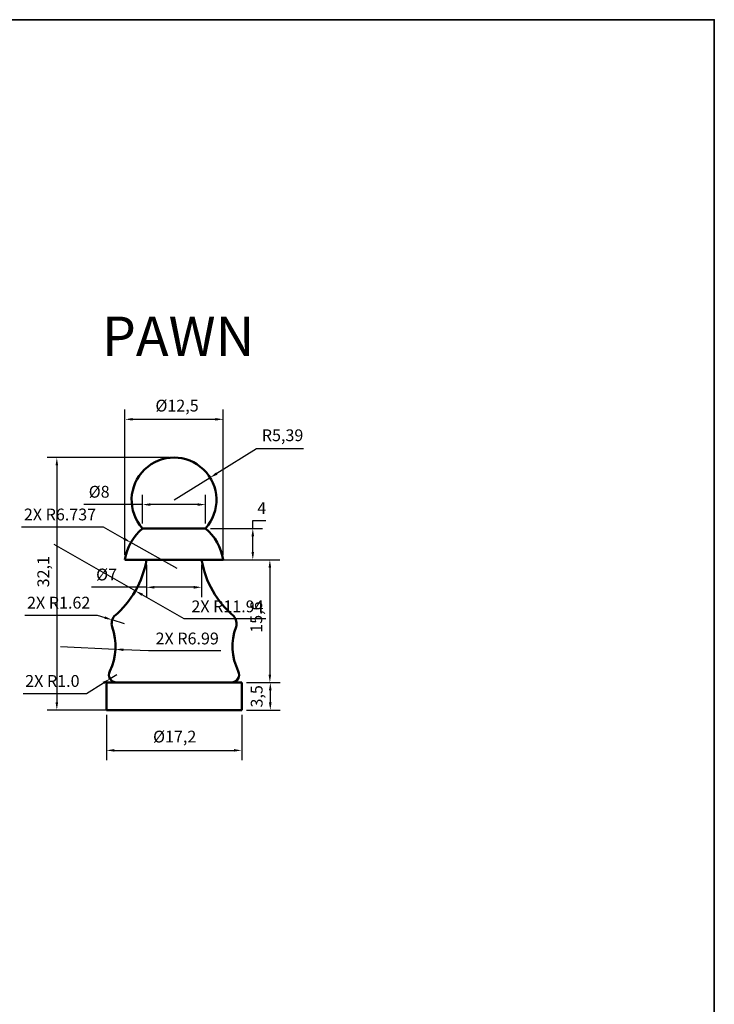
# Model space of a CAD drawing. Units: millimetres. Extents: x 172 to 469, y -14 to 196.
# Tile 5 of 5: x 381 to 469, y 71 to 196. Entities that reach past the tile are written whole.
import ezdxf

# ---------------------------------------------------------------- set-up
doc = ezdxf.new("R2010")
doc.units = ezdxf.units.MM
doc.header["$LTSCALE"] = 0.1
for name, color, linetype, lineweight in [('M-DIMS', 2, 'Continuous', 25), ('M-OUTL', 7, 'Continuous', 50), ('M-TEXT', 3, 'Continuous', 25), ('M-TTLB', 7, 'Continuous', 35)]:
    doc.layers.add(name, color=color, linetype=linetype, lineweight=lineweight)
doc.styles.get("Standard").update_dxf_attribs({"font": 'arial.ttf'})
doc.dimstyles.new('ISO-25', dxfattribs={"dimtxt": 1.5, "dimasz": 1, "dimexe": 1.25, "dimexo": 0.625, "dimtad": 1, "dimtoh": 1, "dimtxsty": 'Standard', "dimcen": 2.5, "dimadec": 0, "dimazin": 0, "dimtfac": 1, "dimtmove": 0, "dimatfit": 3, "dimfxl": 1, "dimarcsym": 0})

# ---------------------------------------------------------------- blocks, each defined once
blk = doc.blocks.new('*D36')
at = {"layer": 'Defpoints', "color": 0, "ltscale": 0.1, "transparency": 16777216}
for p in [(406.97, 145.07), (394.47, 127.21), (406.97, 127.21)]:
    blk.add_point(p, dxfattribs=at)
at = {"layer": 'M-DIMS', "color": 0, "lineweight": -2, "ltscale": 0.1, "transparency": 16777216}
for p, q in [((394.47, 127.84), (394.47, 146.32)), ((406.97, 127.84), (406.97, 146.32)), ((395.47, 145.07), (405.97, 145.07))]:
    blk.add_line(p, q, dxfattribs=at)
at = {"layer": 'M-DIMS', "color": 0, "ltscale": 0.1, "transparency": 16777216}
for points in [[(395.47, 145.24), (395.47, 144.91), (394.47, 145.07)], [(405.97, 145.24), (405.97, 144.91), (406.97, 145.07)]]:
    blk.add_solid(points, dxfattribs=at)
at = {"layer": 'M-DIMS', "color": 0, "ltscale": 0.1, "transparency": 16777216, "insert": (401.1, 146.62), "char_height": 1.5, "attachment_point": 5}
blk.add_mtext('%%C12,5', dxfattribs=at)
blk = doc.blocks.new('*D37')
at = {"layer": 'Defpoints', "color": 0, "ltscale": 0.1, "transparency": 16777216}
for p in [(404.72, 134.23), (396.71, 131.21), (404.72, 131.21)]:
    blk.add_point(p, dxfattribs=at)
at = {"layer": 'M-DIMS', "color": 0, "lineweight": -2, "ltscale": 0.1, "transparency": 16777216}
for p, q in [((396.71, 131.84), (396.71, 135.48)), ((404.72, 131.84), (404.72, 135.48)), ((396.71, 134.23), (389.27, 134.23)), ((403.72, 134.23), (397.71, 134.23))]:
    blk.add_line(p, q, dxfattribs=at)
at = {"layer": 'M-DIMS', "color": 0, "ltscale": 0.1, "transparency": 16777216}
for points in [[(397.71, 134.4), (397.71, 134.07), (396.71, 134.23)], [(403.72, 134.4), (403.72, 134.07), (404.72, 134.23)]]:
    blk.add_solid(points, dxfattribs=at)
at = {"layer": 'M-DIMS', "color": 0, "ltscale": 0.1, "transparency": 16777216, "insert": (391.2, 135.67), "char_height": 1.5, "attachment_point": 5}
blk.add_mtext('%%C8', dxfattribs=at)
blk = doc.blocks.new('*D38')
at = {"layer": 'Defpoints', "color": 0, "ltscale": 0.1, "transparency": 16777216}
for p in [(404.72, 131.21), (404.72, 127.21), (410.73, 127.21)]:
    blk.add_point(p, dxfattribs=at)
at = {"layer": 'M-DIMS', "color": 0, "lineweight": -2, "ltscale": 0.1, "transparency": 16777216}
for p, q in [((410.73, 131.21), (410.73, 132.21)), ((410.73, 132.21), (412.39, 132.21)), ((405.34, 131.21), (411.98, 131.21)), ((410.73, 128.21), (410.73, 130.21)), ((405.34, 127.21), (411.98, 127.21))]:
    blk.add_line(p, q, dxfattribs=at)
at = {"layer": 'M-DIMS', "color": 0, "ltscale": 0.1, "transparency": 16777216}
for points in [[(410.56, 130.21), (410.89, 130.21), (410.73, 131.21)], [(410.56, 128.21), (410.89, 128.21), (410.73, 127.21)]]:
    blk.add_solid(points, dxfattribs=at)
at = {"layer": 'M-DIMS', "color": 0, "ltscale": 0.1, "transparency": 16777216, "insert": (411.87, 133.59), "char_height": 1.5, "attachment_point": 5}
blk.add_mtext('4', dxfattribs=at)
blk = doc.blocks.new('*D39')
at = {"layer": 'Defpoints', "color": 0, "ltscale": 0.1, "transparency": 16777216}
for p in [(397.22, 127.21), (404.22, 127.21), (404.22, 123.72)]:
    blk.add_point(p, dxfattribs=at)
at = {"layer": 'M-DIMS', "color": 0, "lineweight": -2, "ltscale": 0.1, "transparency": 16777216}
for p, q in [((397.22, 126.59), (397.22, 122.47)), ((404.22, 126.59), (404.22, 122.47)), ((397.22, 123.72), (390.21, 123.72)), ((403.22, 123.72), (398.22, 123.72))]:
    blk.add_line(p, q, dxfattribs=at)
at = {"layer": 'M-DIMS', "color": 0, "ltscale": 0.1, "transparency": 16777216}
for points in [[(398.22, 123.89), (398.22, 123.55), (397.22, 123.72)], [(403.22, 123.89), (403.22, 123.55), (404.22, 123.72)]]:
    blk.add_solid(points, dxfattribs=at)
at = {"layer": 'M-DIMS', "color": 0, "ltscale": 0.1, "transparency": 16777216, "insert": (392.14, 125.15), "char_height": 1.5, "attachment_point": 5}
blk.add_mtext('%%C7', dxfattribs=at)
blk = doc.blocks.new('*D40')
at = {"layer": 'Defpoints', "color": 0, "ltscale": 0.1, "transparency": 16777216}
for p in [(400.72, 140.21), (385.82, 108.11), (400.72, 108.11)]:
    blk.add_point(p, dxfattribs=at)
at = {"layer": 'M-DIMS', "color": 0, "lineweight": -2, "ltscale": 0.1, "transparency": 16777216}
for p, q in [((400.09, 140.21), (384.57, 140.21)), ((385.82, 139.21), (385.82, 109.11)), ((400.09, 108.11), (384.57, 108.11))]:
    blk.add_line(p, q, dxfattribs=at)
at = {"layer": 'M-DIMS', "color": 0, "ltscale": 0.1, "transparency": 16777216}
for points in [[(385.65, 139.21), (385.98, 139.21), (385.82, 140.21)], [(385.65, 109.11), (385.98, 109.11), (385.82, 108.11)]]:
    blk.add_solid(points, dxfattribs=at)
at = {"layer": 'M-DIMS', "color": 0, "ltscale": 0.1, "transparency": 16777216, "insert": (384.29, 125.7), "char_height": 1.5, "attachment_point": 5, "rotation": 90}
blk.add_mtext('32,1', dxfattribs=at)
blk = doc.blocks.new('*D41')
at = {"layer": 'Defpoints', "color": 0, "ltscale": 0.1, "transparency": 16777216}
for p in [(408.66, 127.21), (409.32, 111.61), (412.9, 111.61)]:
    blk.add_point(p, dxfattribs=at)
at = {"layer": 'M-DIMS', "color": 0, "lineweight": -2, "ltscale": 0.1, "transparency": 16777216}
for p, q in [((409.29, 127.21), (414.15, 127.21)), ((412.9, 126.21), (412.9, 112.61)), ((409.94, 111.61), (414.15, 111.61))]:
    blk.add_line(p, q, dxfattribs=at)
at = {"layer": 'M-DIMS', "color": 0, "ltscale": 0.1, "transparency": 16777216}
for points in [[(412.73, 126.21), (413.06, 126.21), (412.9, 127.21)], [(412.73, 112.61), (413.06, 112.61), (412.9, 111.61)]]:
    blk.add_solid(points, dxfattribs=at)
at = {"layer": 'M-DIMS', "color": 0, "ltscale": 0.1, "transparency": 16777216, "insert": (411.37, 119.93), "char_height": 1.5, "attachment_point": 5, "rotation": 90}
blk.add_mtext('15,6', dxfattribs=at)
blk = doc.blocks.new('*D42')
at = {"layer": 'Defpoints', "color": 0, "ltscale": 0.1, "transparency": 16777216}
for p in [(392.12, 108.11), (409.32, 108.11), (409.32, 102.99)]:
    blk.add_point(p, dxfattribs=at)
at = {"layer": 'M-DIMS', "color": 0, "lineweight": -2, "ltscale": 0.1, "transparency": 16777216}
for p, q in [((392.12, 107.49), (392.12, 101.74)), ((409.32, 107.49), (409.32, 101.74)), ((393.12, 102.99), (408.32, 102.99))]:
    blk.add_line(p, q, dxfattribs=at)
at = {"layer": 'M-DIMS', "color": 0, "ltscale": 0.1, "transparency": 16777216}
for points in [[(393.12, 103.16), (393.12, 102.83), (392.12, 102.99)], [(408.32, 103.16), (408.32, 102.83), (409.32, 102.99)]]:
    blk.add_solid(points, dxfattribs=at)
at = {"layer": 'M-DIMS', "color": 0, "ltscale": 0.1, "transparency": 16777216, "insert": (400.8, 104.55), "char_height": 1.5, "attachment_point": 5}
blk.add_mtext('%%C17,2', dxfattribs=at)
blk = doc.blocks.new('*D43')
at = {"layer": 'Defpoints', "color": 0, "ltscale": 0.1, "transparency": 16777216}
for p in [(409.32, 111.61), (409.32, 108.11), (412.95, 108.11)]:
    blk.add_point(p, dxfattribs=at)
at = {"layer": 'M-DIMS', "color": 0, "lineweight": -2, "ltscale": 0.1, "transparency": 16777216}
for p, q in [((409.94, 111.61), (414.2, 111.61)), ((412.95, 110.61), (412.95, 109.11)), ((409.94, 108.11), (414.2, 108.11))]:
    blk.add_line(p, q, dxfattribs=at)
at = {"layer": 'M-DIMS', "color": 0, "ltscale": 0.1, "transparency": 16777216}
for points in [[(412.78, 110.61), (413.12, 110.61), (412.95, 111.61)], [(412.78, 109.11), (413.12, 109.11), (412.95, 108.11)]]:
    blk.add_solid(points, dxfattribs=at)
at = {"layer": 'M-DIMS', "color": 0, "ltscale": 0.1, "transparency": 16777216, "insert": (411.42, 109.86), "char_height": 1.5, "attachment_point": 5, "rotation": 90}
blk.add_mtext('3,5', dxfattribs=at)
blk = doc.blocks.new('*D44')
at = {"layer": 'Defpoints', "color": 0, "ltscale": 0.1, "transparency": 16777216}
for p in [(405.3, 137.66), (400.72, 134.82)]:
    blk.add_point(p, dxfattribs=at)
at = {"layer": 'M-DIMS', "color": 0, "lineweight": -2, "ltscale": 0.1, "transparency": 16777216}
for p, q in [((411.21, 141.32), (406.15, 138.19)), ((417.17, 141.32), (411.21, 141.32)), ((400.72, 134.82), (405.3, 137.66))]:
    blk.add_line(p, q, dxfattribs=at)
at = {"layer": 'M-DIMS', "color": 0, "ltscale": 0.1, "transparency": 16777216}
blk.add_solid([(406.06, 138.33), (406.24, 138.04), (405.3, 137.66)], dxfattribs=at)
at = {"layer": 'M-DIMS', "color": 0, "ltscale": 0.1, "transparency": 16777216, "insert": (414.51, 142.85), "char_height": 1.5, "attachment_point": 5}
blk.add_mtext('R5,39', dxfattribs=at)
blk = doc.blocks.new('*D83')
at = {"layer": 'Defpoints', "color": 0, "ltscale": 0.1, "transparency": 16777216}
for p in [(385.44, 129.21), (395.8, 123.27)]:
    blk.add_point(p, dxfattribs=at)
at = {"layer": 'M-DIMS', "color": 0, "lineweight": -2, "ltscale": 0.1, "transparency": 16777216}
for p, q in [((385.44, 129.21), (395.8, 123.27)), ((402.02, 119.71), (396.67, 122.77)), ((412.38, 119.71), (402.02, 119.71))]:
    blk.add_line(p, q, dxfattribs=at)
at = {"layer": 'M-DIMS', "color": 0, "ltscale": 0.1, "transparency": 16777216}
blk.add_solid([(396.75, 122.92), (396.59, 122.63), (395.8, 123.27)], dxfattribs=at)
at = {"layer": 'M-DIMS', "color": 0, "ltscale": 0.1, "transparency": 16777216, "insert": (407.51, 121.1), "char_height": 1.5, "attachment_point": 5}
blk.add_mtext('2X R11.94', dxfattribs=at)
blk = doc.blocks.new('*D84')
at = {"layer": 'Defpoints', "color": 0, "ltscale": 0.1, "transparency": 16777216}
for p in [(395.24, 129.41), (401.11, 126.11)]:
    blk.add_point(p, dxfattribs=at)
at = {"layer": 'M-DIMS', "color": 0, "lineweight": -2, "ltscale": 0.1, "transparency": 16777216}
for p, q in [((381.34, 131.39), (391.72, 131.39)), ((391.72, 131.39), (394.37, 129.9)), ((401.11, 126.11), (395.24, 129.41))]:
    blk.add_line(p, q, dxfattribs=at)
at = {"layer": 'M-DIMS', "color": 0, "ltscale": 0.1, "transparency": 16777216}
blk.add_solid([(394.45, 130.04), (394.29, 129.75), (395.24, 129.41)], dxfattribs=at)
at = {"layer": 'M-DIMS', "color": 0, "ltscale": 0.1, "transparency": 16777216, "insert": (386.22, 132.78), "char_height": 1.5, "attachment_point": 5}
blk.add_mtext('2X R6.737', dxfattribs=at)
blk = doc.blocks.new('*D85')
at = {"layer": 'Defpoints', "color": 0, "ltscale": 0.1, "transparency": 16777216}
for p in [(386.3, 116.19), (393.28, 115.84)]:
    blk.add_point(p, dxfattribs=at)
at = {"layer": 'M-DIMS', "color": 0, "lineweight": -2, "ltscale": 0.1, "transparency": 16777216}
for p, q in [((386.3, 116.19), (393.28, 115.84)), ((397.47, 115.63), (394.28, 115.79)), ((406.68, 115.63), (397.47, 115.63))]:
    blk.add_line(p, q, dxfattribs=at)
at = {"layer": 'M-DIMS', "color": 0, "ltscale": 0.1, "transparency": 16777216}
blk.add_solid([(394.29, 115.95), (394.27, 115.62), (393.28, 115.84)], dxfattribs=at)
at = {"layer": 'M-DIMS', "color": 0, "ltscale": 0.1, "transparency": 16777216, "insert": (402.39, 117.02), "char_height": 1.5, "attachment_point": 5}
blk.add_mtext('2X R6.99', dxfattribs=at)
blk = doc.blocks.new('*D86')
at = {"layer": 'Defpoints', "color": 0, "ltscale": 0.1, "transparency": 16777216}
for p in [(392.86, 119.57), (394.4, 119.08)]:
    blk.add_point(p, dxfattribs=at)
at = {"layer": 'M-DIMS', "color": 0, "lineweight": -2, "ltscale": 0.1, "transparency": 16777216}
for p, q in [((381.76, 120.18), (390.95, 120.18)), ((390.95, 120.18), (391.91, 119.87)), ((394.4, 119.08), (392.86, 119.57))]:
    blk.add_line(p, q, dxfattribs=at)
at = {"layer": 'M-DIMS', "color": 0, "ltscale": 0.1, "transparency": 16777216}
blk.add_solid([(391.96, 120.03), (391.86, 119.72), (392.86, 119.57)], dxfattribs=at)
at = {"layer": 'M-DIMS', "color": 0, "ltscale": 0.1, "transparency": 16777216, "insert": (386.05, 121.57), "char_height": 1.5, "attachment_point": 5}
blk.add_mtext('2X R1.62', dxfattribs=at)
blk = doc.blocks.new('*D87')
at = {"layer": 'Defpoints', "color": 0, "ltscale": 0.1, "transparency": 16777216}
for p in [(392.59, 112.09), (393.44, 112.61)]:
    blk.add_point(p, dxfattribs=at)
at = {"layer": 'M-DIMS', "color": 0, "lineweight": -2, "ltscale": 0.1, "transparency": 16777216}
for p, q in [((389.58, 110.23), (391.74, 111.56)), ((393.44, 112.61), (392.59, 112.09)), ((381.55, 110.23), (389.58, 110.23))]:
    blk.add_line(p, q, dxfattribs=at)
at = {"layer": 'M-DIMS', "color": 0, "ltscale": 0.1, "transparency": 16777216}
blk.add_solid([(391.65, 111.7), (391.83, 111.42), (392.59, 112.09)], dxfattribs=at)
at = {"layer": 'M-DIMS', "color": 0, "ltscale": 0.1, "transparency": 16777216, "insert": (385.25, 111.62), "char_height": 1.5, "attachment_point": 5}
blk.add_mtext('2X R1.0', dxfattribs=at)

msp = doc.modelspace()

# ---------------------------------------------------------------- linework, layer by layer
at = {"layer": 'M-OUTL', "ltscale": 0.1}
for p, q in [((404.7192, 131.2104), (396.7142, 131.2104)), ((406.9667, 127.2104), (394.4667, 127.2104)), ((409.3167, 111.6104), (392.1167, 111.6104)), ((392.1167, 111.6104), (392.1167, 108.1104)), ((409.3167, 108.1104), (409.3167, 111.6104)), ((392.1167, 108.1104), (409.3167, 108.1104))]:
    msp.add_line(p, q, dxfattribs=at)
for points in [[(393.4414, 111.6104, -0.557957), (392.5476, 113.0587, 0.21014457), (392.8325, 118.6782, -0.23002517), (393.117, 120.0607, 0.17802101), (397.2167, 127.2104)], [(407.9919, 111.6104, 0.557957), (408.8858, 113.0587, -0.21014457), (408.6008, 118.6782, 0.23002517), (408.3163, 120.0607, -0.17802101), (404.2167, 127.2104)]]:
    msp.add_lwpolyline(points, format="xyb", dxfattribs=at)
for centre, radius, start, end in [((400.7167, 134.8204), 5.39, 317.951547, 222.048453), ((401.1124, 126.1077), 6.7366, 130.759721, 170.579183), ((400.3209, 126.1077), 6.7366, 9.420817, 49.240279)]:
    msp.add_arc(centre, radius, start, end, dxfattribs=at)
at = {"layer": 'M-TTLB', "ltscale": 0.1}
msp.add_lwpolyline([(172.3921, 195.8665), (469.3921, 195.8665), (469.3921, -14.1335), (172.3921, -14.1335)], close=True, dxfattribs=at)

# ---------------------------------------------------------------- texts
at = {"layer": 'M-TEXT', "ltscale": 0.1, "insert": (379.1411, 158.1383), "char_height": 5, "attachment_point": 1}
msp.add_mtext_dynamic_manual_height_columns('\\pxqc;PAWN', width=44.206943, gutter_width=12.5, heights=[0], dxfattribs=at)

# ---------------------------------------------------------------- dimensions: what is measured, and where the dimension line sits
at = {"layer": 'M-DIMS', "ltscale": 0.1}
for base, p1, p2, picture, middle in [((406.9667, 145.0726), (394.4667, 127.2104), (406.9667, 127.2104), '*D36', (401.1016, 145.0726)), ((404.719161, 134.234382), (396.714163, 131.210354), (404.719161, 131.210353), '*D37', (391.199993, 134.234382)), ((404.2167, 123.7192), (397.2167, 127.2104), (404.2167, 127.2104), '*D39', (392.1438, 123.7192)), ((409.3167, 102.9945), (392.1167, 108.1104), (409.3167, 108.1104), '*D42', (400.7965, 102.9945))]:
    dim = msp.add_linear_dim(base=base, p1=p1, p2=p2, text='%%C<>', dimstyle='ISO-25', override={"dimclrd": 0, "dimclre": 0, "dimclrt": 0}, dxfattribs=at)
    dim.commit()
    dim.dimension.update_dxf_attribs({"geometry": picture, "text_midpoint": middle, "dimtype": 160})
dim = msp.add_radius_dim(center=(400.7167, 134.8204), mpoint=(405.2989, 137.6585), dimstyle='ISO-25', override={"dimclrd": 0, "dimclre": 0, "dimclrt": 0}, dxfattribs=at)
dim.commit()
dim.dimension.update_dxf_attribs({"geometry": '*D44', "text_midpoint": (414.5072, 141.3226), "dimtype": 164})
for base, p1, p2, picture, middle in [((385.8181, 108.1104), (400.7167, 140.2104), (400.7167, 108.1104), '*D40', (385.8181, 125.6953)), ((410.726, 127.2104), (404.7192, 131.2104), (404.7192, 127.2104), '*D38', (411.8698, 132.2104)), ((412.8973, 111.6104), (408.6601, 127.2104), (409.3167, 111.6104), '*D41', (412.8973, 119.9266)), ((412.9486, 108.1104), (409.3167, 111.6104), (409.3167, 108.1104), '*D43', (412.9486, 109.8604))]:
    dim = msp.add_linear_dim(base=base, p1=p1, p2=p2, angle=90, dimstyle='ISO-25', override={"dimclrd": 0, "dimclre": 0, "dimclrt": 0}, dxfattribs=at)
    dim.commit()
    dim.dimension.update_dxf_attribs({"geometry": picture, "text_midpoint": middle, "dimtype": 160})
for center, mpoint, override, picture, middle in [((401.1124, 126.1077), (395.2395, 129.4077), {"dimdec": 3, "dimlfac": 1, "dimrnd": 0, "dimzin": 0, "dimdsep": 46, "dimlunit": 2}, '*D84', (386.2177, 131.3878)), ((385.4445, 129.2104), (395.8033, 123.2708), {"dimdec": 2, "dimlfac": 1, "dimrnd": 0, "dimzin": 0, "dimdsep": 46, "dimlunit": 2}, '*D83', (407.5135, 119.7071)), ((386.3, 116.1925), (393.2805, 115.839), {"dimdec": 2, "dimlfac": 1, "dimrnd": 0, "dimzin": 0, "dimdsep": 46, "dimlunit": 2}, '*D85', (397.4688, 115.6269))]:
    dim = msp.add_radius_dim(center=center, mpoint=mpoint, text='2X <>', dimstyle='ISO-25', override=override, dxfattribs=at)
    dim.commit()
    dim.dimension.update_dxf_attribs({"geometry": picture, "text_midpoint": middle, "dimtype": 164})
for center, mpoint, override, picture, middle in [((394.3978, 119.0766), (392.8595, 119.569), {"dimdec": 2, "dimlfac": 1, "dimrnd": 0, "dimzin": 0, "dimdsep": 46, "dimlunit": 2}, '*D86', (386.0471, 121.5696)), ((393.4414, 112.6104), (392.5904, 112.0852), {"dimdec": 1, "dimlfac": 1, "dimrnd": 0, "dimzin": 0, "dimdsep": 46, "dimlunit": 2}, '*D87', (385.255, 111.6212))]:
    dim = msp.add_radius_dim(center=center, mpoint=mpoint, text='2X <>', dimstyle='ISO-25', override=override, dxfattribs=at)
    dim.commit()
    dim.dimension.update_dxf_attribs({"geometry": picture, "text_midpoint": middle})

doc.saveas('drawing.dxf')
